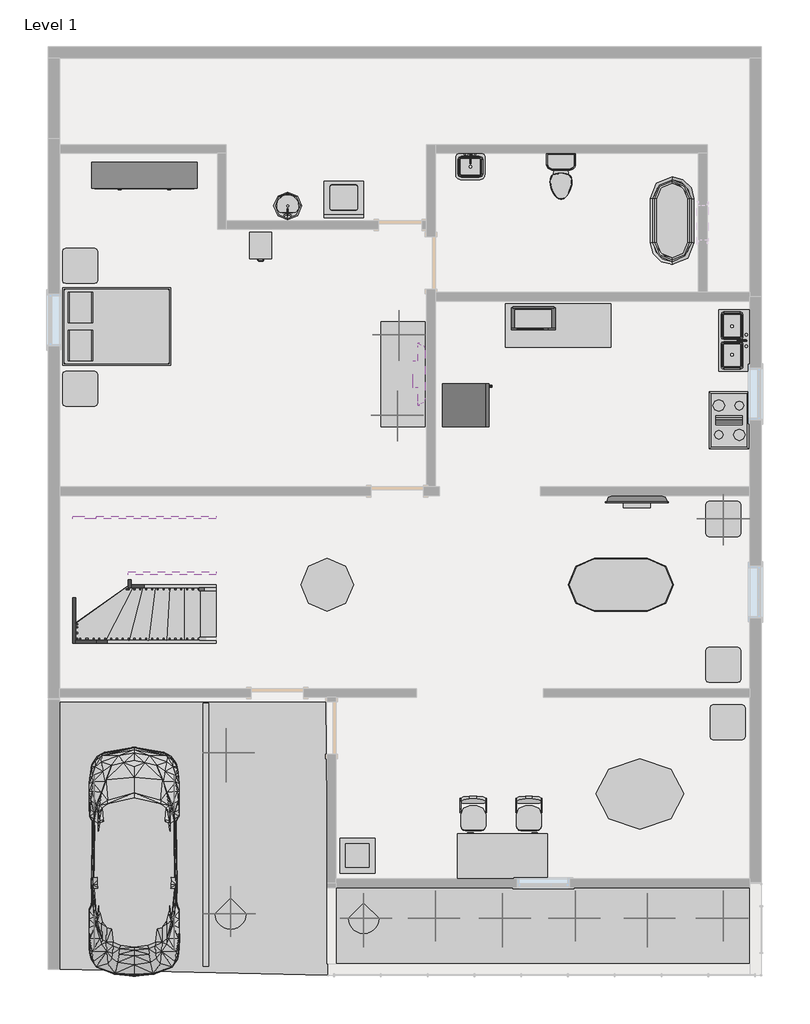
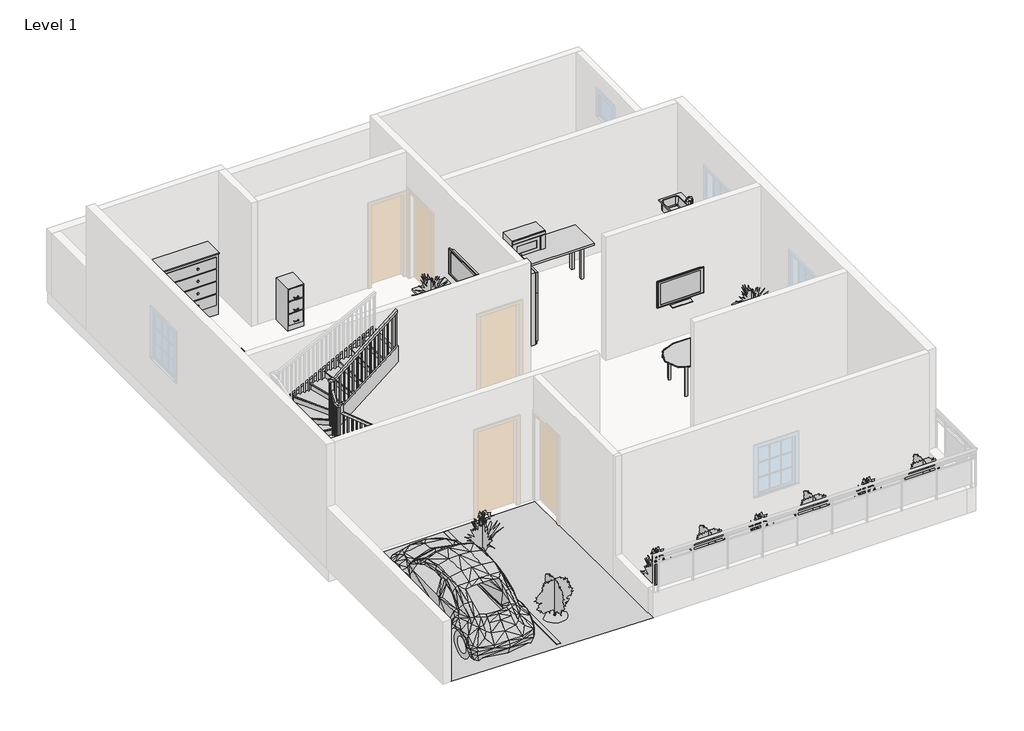
# One storey, part 3 of 3: 19 furniture elements, 11 geographic elements, 8 members, 8 proxies, 7 flow terminals, 1 railing, 1 stair flight.
# Revit data of these elements (continued)
# Element 55 (IfcStairFlight, "2\" Tread 1\" Nosing 1/4\" Riser") (continued)
#   Phase Created = New Construction
# Materials
#   "Steel, Chrome Plated": class "Metal", colour RGB 17 17 17, transparency 0, Description = "Chromiuim plated steel", Cost = 0
#   "Steel, Polished": class "Metal", colour RGB 57 57 57, transparency 0, Description = "Polished steel", Cost = 0
#   "Laminate, Ivory, Matte": class "Plastic", colour RGB 247 247 239, transparency 0, Description = "Plastic Laminate - Ivory, Matte", Cost = 0
#   "Steel, Paint Finish, Ivory, Glossy": class "Metal", colour RGB 247 247 239, transparency 0, Description = "Steel, paint finish, ivory, glossy", Cost = 0
#   "Steel, Paint Finish, Ivory, Matte": class "Metal", colour RGB 247 247 239, transparency 0, Description = "Steel, paint finish, ivory, matte", Cost = 0
#   "Porcelain, Linen": class "Ceramic", colour RGB 249 239 230, transparency 0, Description = "Porcelain, linen", Cost = 0
#   "Laminate, Linen, Matte": class "Plastic", colour RGB 249 239 230, transparency 0, Description = "Plastic Laminate - Linen, Matte", Cost = 0
#   "Porcelain, Ivory": class "Ceramic", colour RGB 247 247 239, transparency 0, Description = "Porcelain, ivory", Cost = 0
#   "Birch": class "Wood", colour RGB 224 178 126, transparency 0, Description = "Betula Alleghaniensis", Cost = 0
#   "Linen, White": class "Textile", colour RGB 247 247 239, transparency 0, Description = "Linen, white", Cost = 0
#   "Cherry": class "Wood", colour RGB 226 177 128, transparency 0, Description = "Prunus Serotina", Cost = 0
#   "Laminate - Ivory, Glossy": colour RGB 247 247 239, transparency 0
#   "Linen, Beige": class "Textile", colour RGB 249 239 230, transparency 0, Description = "Linen, beige", Cost = 0
#   "Steel, Paint Finish, Dark Gray, Matte": class "Metal", colour RGB 0 0 0, transparency 0, Description = "Steel, paint finish, dark gray, matte", Cost = 0
#   "Glass - Clear, Grey": class "Glass", colour RGB 252 255 255, transparency 0.64
#   "Pine": class "Wood", colour RGB 223 192 134, transparency 0, Description = "Pinus Echinata", Cost = 0
#   "Glass": class "Glass", colour RGB 0 128 192, transparency 0.75, Description = "Soda Lime Glass", Cost = 0
#   "Parking Stripe": class "Paint", colour RGB 250 250 91, transparency 0
#   "TV - Black": colour RGB 49 49 49, transparency 0
#   "TV - Glass": colour RGB 157 157 157, transparency 0.9
#   "TV - Screen": colour RGB 0 0 0, transparency 0
